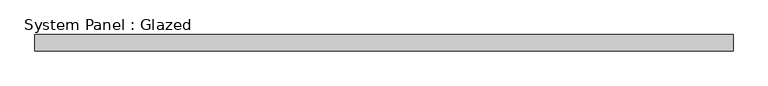
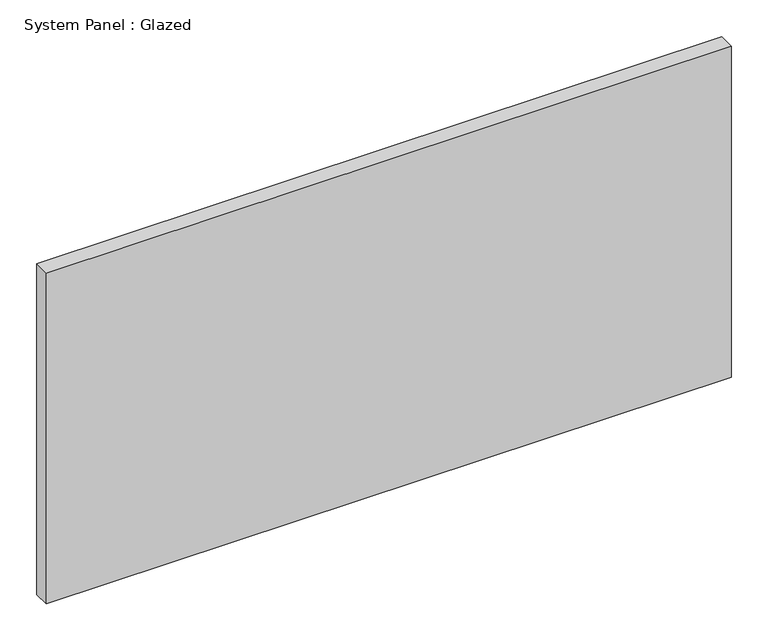
"""IFC4 building model written with IfcOpenShell, lengths in millimetres: plate geometry, System Panel : Glazed."""

from ifc_helpers import new_model, si_unit, origin, origin_with_axes, place, context, project, spatial, polyline, outline, extrude, source, transform, mapped, element, save


def system_panel_glazed_e581be51(model_context):
    return source(origin(), model_context, "Body", "SweptSolid", [
        extrude(outline(polyline([(534.4583334, 19.05), (-534.4583334, 19.05), (-534.4583334, 44.45), (534.4583334, 44.45), (534.4583334, 19.05)])), origin_with_axes(), (0.0, 0.0, 1.0), 546.1),
    ])


if __name__ == "__main__":
    model = new_model("IFC4")
    model_context = context("Model", 3, world=origin())
    ifc_project = project(units=[si_unit("LENGTHUNIT", "METRE", prefix="MILLI")], contexts=[model_context])
    site = spatial("IfcSite", under=ifc_project)
    building = spatial("IfcBuilding", under=site)
    placement = place(None, origin())
    system_panel_glazed_shape = system_panel_glazed_e581be51(model_context)
    element("IfcPlate", 1, ObjectType="System Panel : Glazed", at=placement, inside=building, context=model_context, shape_type="MappedRepresentation", body=[
        mapped(system_panel_glazed_shape, transform((0.0, 0.0, 0.0), x_axis=(1.0, 0.0, 0.0), y_axis=(0.0, 1.0, 0.0), z_axis=(0.0, 0.0, 1.0))),
    ])
    save(model, "model.ifc")

# Revit data of these elements
# Type "System Panel : Glazed"
#   Construction Type Id = "GSP4R"
#   Analytic Construction = "1/8 in Pilkington single glazing"
#   Visual Light Transmittance = 0.9
#   Solar Heat Gain Coefficient = 0.86
#   Heat Transfer Coefficient (U) = 1.18115 BTU/(h·ft²·°F)
#   Define Thermal Properties by = 1
# Element 1 (IfcPlate, "System Panel : Glazed")
#   Materials on its faces: "Glass"
# Materials
#   "Glass": class "Glass", colour RGB 0 128 192, transparency 0.75, Description = "Soda Lime Glass", Cost = 0
